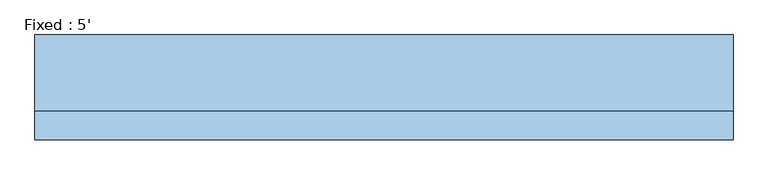
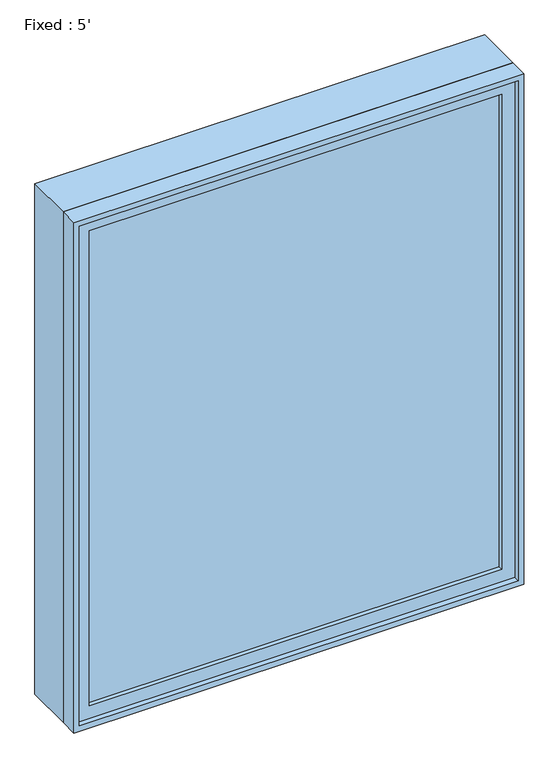
"""IFC4 building model written with IfcOpenShell, lengths in millimetres: window geometry, Fixed : 5'."""

from ifc_helpers import new_model, si_unit, frame, origin, place, context, project, spatial, polyline, outline, extrude, source, transform, mapped, element, save


def fixed_5_6e519979(model_context):
    return source(origin(), model_context, "Body", "SweptSolid", [
        extrude(outline(polyline([(660.4, -66.675), (660.4, -79.375), (-736.6, -79.375), (-736.6, -66.675), (660.4, -66.675)])), frame((0.0, 0.0, 368.3), z_axis=(0.0, 0.0, 1.0), x_axis=(1.0, 0.0, 0.0)), (0.0, 0.0, 1.0), 1701.8),
        extrude(outline(polyline([(2114.55, -781.05), (323.85, -781.05), (323.85, 704.85), (2114.55, 704.85), (2114.55, -781.05)]), holes=[polyline([(2070.1, -736.6), (2070.1, 660.4), (368.3, 660.4), (368.3, -736.6), (2070.1, -736.6)])]), frame((0.0, -95.25, 0.0), z_axis=(0.0, 1.0, 0.0), x_axis=(0.0, 0.0, 1.0)), (0.0, 0.0, 1.0), 44.45),
        extrude(outline(polyline([(2133.6, -800.1), (304.8, -800.1), (304.8, 723.9), (2133.6, 723.9), (2133.6, -800.1)]), holes=[polyline([(2101.85, -768.35), (2101.85, 692.15), (336.55, 692.15), (336.55, -768.35), (2101.85, -768.35)])]), frame((0.0, -50.8, 0.0), z_axis=(0.0, 1.0, 0.0), x_axis=(0.0, 0.0, 1.0)), (0.0, 0.0, 1.0), 165.1),
        extrude(outline(polyline([(2133.6, 723.9), (2133.6, -800.1), (304.8, -800.1), (304.8, 723.9), (2133.6, 723.9)]), holes=[polyline([(2114.55, 704.85), (323.85, 704.85), (323.85, -781.05), (2114.55, -781.05), (2114.55, 704.85)])]), frame((0.0, -114.3, 0.0), z_axis=(0.0, 1.0, 0.0), x_axis=(0.0, 0.0, 1.0)), (0.0, 0.0, 1.0), 63.5),
    ])


if __name__ == "__main__":
    model = new_model("IFC4")
    model_context = context("Model", 3, world=origin())
    ifc_project = project(units=[si_unit("LENGTHUNIT", "METRE", prefix="MILLI")], contexts=[model_context])
    site = spatial("IfcSite", under=ifc_project)
    building = spatial("IfcBuilding", under=site)
    placement = place(None, origin())
    fixed_5_shape = fixed_5_6e519979(model_context)
    element("IfcWindow", 1, ObjectType="Fixed : 5'", at=placement, inside=building, context=model_context, shape_type="MappedRepresentation", body=[
        mapped(fixed_5_shape, transform((0.0, 0.0, 0.0), x_axis=(1.0, 0.0, 0.0), y_axis=(0.0, 1.0, 0.0), z_axis=(0.0, 0.0, 1.0))),
    ])
    save(model, "model.ifc")

# Revit data of these elements
# Type "Fixed : 5'"
#   Type Mark = "16"
#   Construction Type Id = "GSP4R"
#   Assembly Code = "B2020100"
#   Analytic Construction = "1/8 in Pilkington single glazing"
#   Visual Light Transmittance = 0.9
#   Solar Heat Gain Coefficient = 0.78
#   Heat Transfer Coefficient (U) = 0.6496 BTU/(h·ft²·°F)
#   Height = 6' - 0"
#   Default Sill Height = 1' - 0"
#   Width = 5' - 0"
#   Window Inset = 0' - 0 3/4"
#   Define Thermal Properties by = 1
#   Glass Pane Material = Glass
#   Sash Material = Sash
#   Wall Closure = (empty or 0)
# Element 1 (IfcWindow, "Fixed : 5'")
#   Materials on its faces: "Sash", "Glass"
# Materials
#   "Glass": class "Glass", colour RGB 0 128 192, transparency 0.75, Description = "Soda Lime Glass", Cost = 0
#   "Sash": class "Wood", colour RGB 224 178 126, transparency 0
